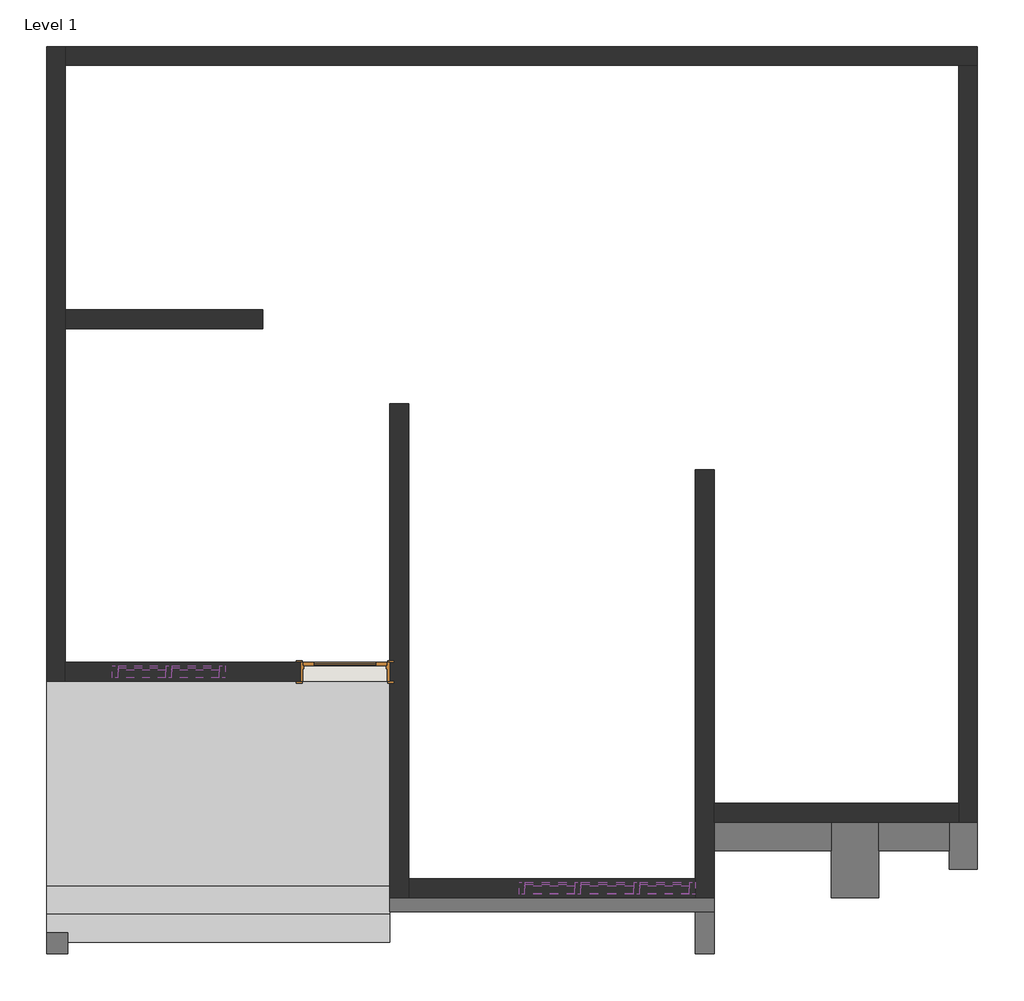
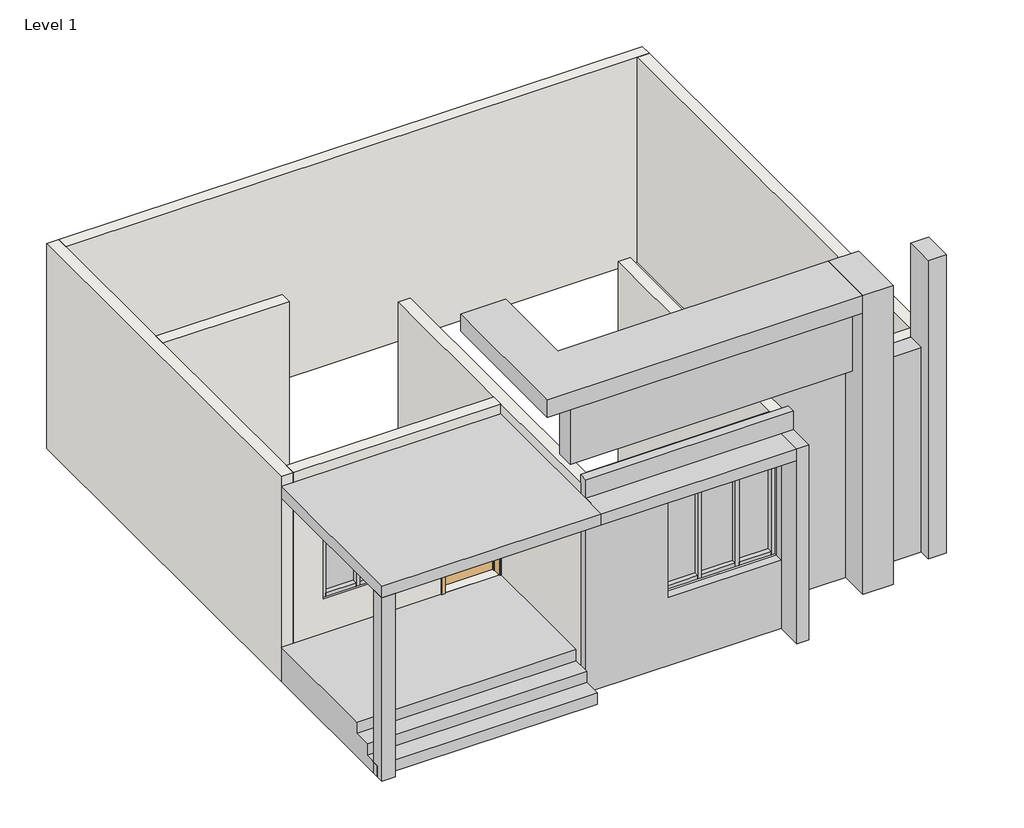
# One storey: 17 members, 9 walls, 5 plates, 1 door, 1 proxy.
"""IFC4 building model written with IfcOpenShell, lengths in millimetres."""

from ifc_helpers import new_model, si_unit, frame, origin, origin_with_axes, place, context, project, spatial, polyline, outline, extrude, faceted_brep, transform, mapped, element, save
from components import generic_models_1_generic_models_1_adbbf048, door_8805718f, member_81de2198, member_d73967ec, member_c8189573, member_bdc0ab2a, member_0b7646a3, system_panel_glazed_2339bcea, system_panel_glazed_76ec949d, system_panel_glazed_5c6be660

model = new_model("IFC4")

# Units and contexts
model_context = context("Model", 3, world=origin())
ifc_project = project(units=[si_unit("LENGTHUNIT", "METRE", prefix="MILLI")], contexts=[model_context])

# Site, building, storey
site = spatial("IfcSite", under=ifc_project)
building = spatial("IfcBuilding", under=site)
storey = spatial("IfcBuildingStorey", under=building, Name="Level 1", Elevation=0.0)

# Proxy
placement = place(None, origin())
generic_models_1_generic_models_1_shape = generic_models_1_generic_models_1_adbbf048(model_context)
element("IfcBuildingElementProxy", 1, Name="Generic Models 1 : Generic Models 1", ObjectType="Generic Models 1 : Generic Models 1", at=placement, inside=storey, context=model_context, shape_type="MappedRepresentation", body=[
    mapped(generic_models_1_generic_models_1_shape, transform((0.0, 0.0, 0.0), x_axis=(1.0, 0.0, 0.0), y_axis=(0.0, 1.0, 0.0), z_axis=(0.0, 0.0, 1.0))),
])

# Door
door_shape = door_8805718f(model_context)
element("IfcDoor", 2, ObjectType="Door-Interior-Single-1_Panel-Wood : 36\" x 96\"", at=placement, inside=storey, context=model_context, shape_type="MappedRepresentation", body=[
    mapped(door_shape, transform((-5421.359401, 7373.8183441, 609.6), x_axis=(1.0, 0.0, 0.0), y_axis=(0.0, 1.0, 0.0), z_axis=(0.0, 0.0, 1.0))),
])

# Members
member_shape = member_81de2198(model_context)
element("IfcMember", 3, ObjectType="Rectangular Mullion : 2.5\" x 5\" rectangular", at=placement, inside=storey, context=model_context, shape_type="MappedRepresentation", body=[
    mapped(member_shape, transform((-3478.259401, 5033.8433441, 3073.4), x_axis=(0.0, 0.0, 1.0), y_axis=(0.0, 1.0, 0.0), z_axis=(-1.0, 0.0, 0.0))),
])
element("IfcMember", 4, ObjectType="Rectangular Mullion : 2.5\" x 5\" rectangular", at=placement, inside=storey, context=model_context, shape_type="MappedRepresentation", body=[
    mapped(member_shape, transform((-2240.009401, 5033.8433441, 3073.4), x_axis=(0.0, 0.0, 1.0), y_axis=(0.0, 1.0, 0.0), z_axis=(-1.0, 0.0, 0.0))),
])
element("IfcMember", 5, ObjectType="Rectangular Mullion : 2.5\" x 5\" rectangular", at=placement, inside=storey, context=model_context, shape_type="MappedRepresentation", body=[
    mapped(member_shape, transform((-1700.259401, 5033.8433441, 1219.2), x_axis=(0.0, 0.0, -1.0), y_axis=(0.0, 1.0, 0.0), z_axis=(1.0, 0.0, 0.0))),
])
element("IfcMember", 6, ObjectType="Rectangular Mullion : 2.5\" x 5\" rectangular", at=placement, inside=storey, context=model_context, shape_type="MappedRepresentation", body=[
    mapped(member_shape, transform((-2938.509401, 5033.8433441, 1219.2), x_axis=(0.0, 0.0, -1.0), y_axis=(0.0, 1.0, 0.0), z_axis=(1.0, 0.0, 0.0))),
])
member_2_shape = member_d73967ec(model_context)
element("IfcMember", 7, ObjectType="Rectangular Mullion : 2.5\" x 5\" rectangular", at=placement, inside=storey, context=model_context, shape_type="MappedRepresentation", body=[
    mapped(member_2_shape, transform((-2906.759401, 5033.8433441, 1219.2), x_axis=(-1.0, 0.0, 0.0), y_axis=(0.0, 1.0, 0.0), z_axis=(0.0, 0.0, -1.0))),
])
element("IfcMember", 8, ObjectType="Rectangular Mullion : 2.5\" x 5\" rectangular", at=placement, inside=storey, context=model_context, shape_type="MappedRepresentation", body=[
    mapped(member_2_shape, transform((-2271.759401, 5033.8433441, 1219.2), x_axis=(-1.0, 0.0, 0.0), y_axis=(0.0, 1.0, 0.0), z_axis=(0.0, 0.0, -1.0))),
])
member_3_shape = member_c8189573(model_context)
element("IfcMember", 9, ObjectType="Rectangular Mullion : 2.5\" x 5\" rectangular", at=placement, inside=storey, context=model_context, shape_type="MappedRepresentation", body=[
    mapped(member_3_shape, transform((-2303.509401, 5033.8433441, 1219.2), x_axis=(0.0, 0.0, -1.0), y_axis=(0.0, 1.0, 0.0), z_axis=(1.0, 0.0, 0.0))),
])
element("IfcMember", 10, ObjectType="Rectangular Mullion : 2.5\" x 5\" rectangular", at=placement, inside=storey, context=model_context, shape_type="MappedRepresentation", body=[
    mapped(member_3_shape, transform((-2875.009401, 5033.8433441, 3073.4), x_axis=(0.0, 0.0, 1.0), y_axis=(0.0, 1.0, 0.0), z_axis=(-1.0, 0.0, 0.0))),
])
member_4_shape = member_bdc0ab2a(model_context)
element("IfcMember", 11, ObjectType="Rectangular Mullion : 2.5\" x 5\" rectangular", at=placement, inside=storey, context=model_context, shape_type="MappedRepresentation", body=[
    mapped(member_4_shape, transform((-1636.759401, 5033.8433441, 3073.4), x_axis=(1.0, 0.0, 0.0), y_axis=(0.0, 1.0, 0.0), z_axis=(0.0, 0.0, 1.0))),
])
element("IfcMember", 12, ObjectType="Rectangular Mullion : 2.5\" x 5\" rectangular", at=placement, inside=storey, context=model_context, shape_type="MappedRepresentation", body=[
    mapped(member_4_shape, transform((-3541.759401, 5033.8433441, 1219.2), x_axis=(-1.0, 0.0, 0.0), y_axis=(0.0, 1.0, 0.0), z_axis=(0.0, 0.0, -1.0))),
])
member_5_shape = member_0b7646a3(model_context)
element("IfcMember", 13, ObjectType="Rectangular Mullion : 2.5\" x 5\" rectangular", at=placement, inside=storey, context=model_context, shape_type="MappedRepresentation", body=[
    mapped(member_5_shape, transform((-6780.259401, 7370.6433441, 3073.4), x_axis=(0.0, 0.0, 1.0), y_axis=(0.0, -1.0, 0.0), z_axis=(1.0, 0.0, 0.0))),
])
element("IfcMember", 14, ObjectType="Rectangular Mullion : 2.5\" x 5\" rectangular", at=placement, inside=storey, context=model_context, shape_type="MappedRepresentation", body=[
    mapped(member_5_shape, transform((-7358.109401, 7370.6433441, 3073.4), x_axis=(0.0, 0.0, 1.0), y_axis=(0.0, -1.0, 0.0), z_axis=(1.0, 0.0, 0.0))),
])
element("IfcMember", 15, ObjectType="Rectangular Mullion : 2.5\" x 5\" rectangular", at=placement, inside=storey, context=model_context, shape_type="MappedRepresentation", body=[
    mapped(member_5_shape, transform((-7872.459401, 7370.6433441, 1219.2), x_axis=(0.0, 0.0, -1.0), y_axis=(0.0, -1.0, 0.0), z_axis=(-1.0, 0.0, 0.0))),
])
element("IfcMember", 16, ObjectType="Rectangular Mullion : 2.5\" x 5\" rectangular", at=placement, inside=storey, context=model_context, shape_type="MappedRepresentation", body=[
    mapped(member_5_shape, transform((-7294.609401, 7370.6433441, 1219.2), x_axis=(0.0, 0.0, -1.0), y_axis=(0.0, -1.0, 0.0), z_axis=(-1.0, 0.0, 0.0))),
])
element("IfcMember", 17, ObjectType="Rectangular Mullion : 2.5\" x 5\" rectangular", at=placement, inside=storey, context=model_context, shape_type="MappedRepresentation", body=[
    mapped(member_2_shape, transform((-7326.359401, 7370.6433441, 1219.2), x_axis=(1.0, 0.0, 0.0), y_axis=(0.0, -1.0, 0.0), z_axis=(0.0, 0.0, -1.0))),
])
element("IfcMember", 18, ObjectType="Rectangular Mullion : 2.5\" x 5\" rectangular", at=placement, inside=storey, context=model_context, shape_type="MappedRepresentation", body=[
    mapped(member_4_shape, transform((-7935.959401, 7370.6433441, 3073.4), x_axis=(-1.0, 0.0, 0.0), y_axis=(0.0, -1.0, 0.0), z_axis=(0.0, 0.0, 1.0))),
])
element("IfcMember", 19, ObjectType="Rectangular Mullion : 2.5\" x 5\" rectangular", at=placement, inside=storey, context=model_context, shape_type="MappedRepresentation", body=[
    mapped(member_4_shape, transform((-6716.759401, 7370.6433441, 1219.2), x_axis=(1.0, 0.0, 0.0), y_axis=(0.0, -1.0, 0.0), z_axis=(0.0, 0.0, -1.0))),
])

# Plates
system_panel_glazed_shape = system_panel_glazed_2339bcea(model_context)
element("IfcPlate", 20, ObjectType="System Panel : Glazed", at=placement, inside=storey, context=model_context, shape_type="MappedRepresentation", body=[
    mapped(system_panel_glazed_shape, transform((-1970.134401, 5033.8433441, 1282.7), x_axis=(-1.0, 0.0, 0.0), y_axis=(0.0, -1.0, 0.0), z_axis=(0.0, 0.0, 1.0))),
])
element("IfcPlate", 21, ObjectType="System Panel : Glazed", at=placement, inside=storey, context=model_context, shape_type="MappedRepresentation", body=[
    mapped(system_panel_glazed_shape, transform((-3208.384401, 5033.8433441, 1282.7), x_axis=(-1.0, 0.0, 0.0), y_axis=(0.0, -1.0, 0.0), z_axis=(0.0, 0.0, 1.0))),
])
system_panel_glazed_2_shape = system_panel_glazed_76ec949d(model_context)
element("IfcPlate", 22, ObjectType="System Panel : Glazed", at=placement, inside=storey, context=model_context, shape_type="MappedRepresentation", body=[
    mapped(system_panel_glazed_2_shape, transform((-2589.259401, 5033.8433441, 1282.7), x_axis=(-1.0, 0.0, 0.0), y_axis=(0.0, -1.0, 0.0), z_axis=(0.0, 0.0, 1.0))),
])
system_panel_glazed_3_shape = system_panel_glazed_5c6be660(model_context)
element("IfcPlate", 23, ObjectType="System Panel : Glazed", at=placement, inside=storey, context=model_context, shape_type="MappedRepresentation", body=[
    mapped(system_panel_glazed_3_shape, transform((-7615.284401, 7370.6433441, 1282.7), x_axis=(1.0, 0.0, 0.0), y_axis=(0.0, 1.0, 0.0), z_axis=(0.0, 0.0, 1.0))),
])
element("IfcPlate", 24, ObjectType="System Panel : Glazed", at=placement, inside=storey, context=model_context, shape_type="MappedRepresentation", body=[
    mapped(system_panel_glazed_3_shape, transform((-7037.434401, 7370.6433441, 1282.7), x_axis=(1.0, 0.0, 0.0), y_axis=(0.0, 1.0, 0.0), z_axis=(0.0, 0.0, 1.0))),
])

# Walls
element("IfcWall", 25, ObjectType="9\" wall", at=placement, inside=storey, context=model_context, shape_type="Brep", body=[
    faceted_brep([(-8647.159401, 14127.0433441, 0.0), (-8647.159401, 7269.0433441, 0.0), (-8647.159401, 7269.0433441, 3657.6), (-8647.159401, 14127.0433441, 3657.6), (-8443.959401, 14127.0433441, 0.0), (-8443.959401, 14127.0433441, 3657.6), (-8443.959401, 13923.8433441, 3657.6), (-8443.959401, 11282.2433441, 3657.6), (-8443.959401, 11079.0433441, 3657.6), (-8443.959401, 7472.2433441, 3657.6), (-8443.959401, 7269.0433441, 3657.6), (-8443.959401, 7269.0433441, 0.0), (-8443.959401, 7472.2433441, 0.0), (-8443.959401, 11079.0433441, 0.0), (-8443.959401, 11282.2433441, 0.0), (-8443.959401, 13923.8433441, 0.0)], [[[0, 1, 2, 3]], [[4, 5, 6, 7, 8, 9, 10, 11, 12, 13, 14, 15]], [[1, 0, 4, 15, 14, 13, 12, 11]], [[3, 2, 10, 9, 8, 7, 6, 5]], [[2, 1, 11, 10]], [[0, 3, 5, 4]]]),
])
element("IfcWall", 26, ObjectType="9\" wall", at=placement, inside=storey, context=model_context, shape_type="SweptSolid", body=[
    extrude(outline(polyline([(-6310.359401, 11079.0433441), (-8443.959401, 11079.0433441), (-8443.959401, 11282.2433441), (-6310.359401, 11282.2433441), (-6310.359401, 11079.0433441)])), origin_with_axes(), (0.0, 0.0, 1.0), 3657.6),
])
element("IfcWall", 27, ObjectType="9\" wall", at=placement, inside=storey, context=model_context, shape_type="SweptSolid", body=[
    extrude(outline(polyline([(0.0, -8443.959401), (0.0, -4938.759401), (609.6, -4938.759401), (609.6, -5903.959401), (3073.4, -5903.959401), (3073.4, -4938.759401), (3657.6, -4938.759401), (3657.6, -8443.959401), (0.0, -8443.959401)]), holes=[polyline([(1219.2, -7935.959401), (3073.4, -7935.959401), (3073.4, -6716.759401), (1219.2, -6716.759401), (1219.2, -7935.959401)])]), frame((0.0, 7269.0433441, 0.0), z_axis=(0.0, 1.0, 0.0), x_axis=(0.0, 0.0, 1.0)), (0.0, 0.0, 1.0), 203.2),
])
element("IfcWall", 28, ObjectType="9\" wall", at=placement, inside=storey, context=model_context, shape_type="Brep", body=[
    faceted_brep([(-8443.959401, 13923.8433441, 0.0), (1208.040599, 13923.8433441, 0.0), (1411.240599, 13923.8433441, 0.0), (1411.240599, 13923.8433441, 3657.6), (1208.040599, 13923.8433441, 3657.6), (-8443.959401, 13923.8433441, 3657.6), (-8443.959401, 14127.0433441, 0.0), (-8443.959401, 14127.0433441, 3657.6), (1411.240599, 14127.0433441, 3657.6), (1411.240599, 14127.0433441, 0.0)], [[[0, 1, 2, 3, 4, 5]], [[6, 7, 8, 9]], [[2, 1, 0, 6, 9]], [[5, 4, 3, 8, 7]], [[0, 5, 7, 6]], [[3, 2, 9, 8]]]),
])
element("IfcWall", 29, ObjectType="9\" wall", at=placement, inside=storey, context=model_context, shape_type="Brep", body=[
    faceted_brep([(1208.040599, 13923.8433441, 0.0), (1208.040599, 5948.2433441, 0.0), (1208.040599, 5745.0433441, 0.0), (1208.040599, 5745.0433441, 3657.6), (1208.040599, 5948.2433441, 3657.6), (1208.040599, 13923.8433441, 3657.6), (1411.240599, 13923.8433441, 0.0), (1411.240599, 13923.8433441, 3657.6), (1411.240599, 5745.0433441, 3657.6), (1411.240599, 5745.0433441, 0.0)], [[[0, 1, 2, 3, 4, 5]], [[6, 7, 8, 9]], [[2, 1, 0, 6, 9]], [[5, 4, 3, 8, 7]], [[0, 5, 7, 6]], [[3, 2, 9, 8]]]),
])
element("IfcWall", 30, ObjectType="9\" wall", at=placement, inside=storey, context=model_context, shape_type="SweptSolid", body=[
    extrude(outline(polyline([(-1433.559401, 5948.2433441), (1208.040599, 5948.2433441), (1208.040599, 5745.0433441), (-1433.559401, 5745.0433441), (-1433.559401, 5948.2433441)])), origin_with_axes(), (0.0, 0.0, 1.0), 3657.6),
])
element("IfcWall", 31, ObjectType="9\" wall", at=placement, inside=storey, context=model_context, shape_type="Brep", body=[
    faceted_brep([(-1433.559401, 4932.2433441, 0.0), (-1433.559401, 5745.0433441, 0.0), (-1433.559401, 5948.2433441, 0.0), (-1433.559401, 9555.0433441, 0.0), (-1433.559401, 9555.0433441, 3657.6), (-1433.559401, 5948.2433441, 3657.6), (-1433.559401, 5745.0433441, 3657.6), (-1433.559401, 4932.2433441, 3657.6), (-1636.759401, 4932.2433441, 0.0), (-1636.759401, 4932.2433441, 1219.2), (-1636.759401, 4932.2433441, 3073.4), (-1636.759401, 4932.2433441, 3657.6), (-1636.759401, 5135.4433441, 3657.6), (-1636.759401, 9555.0433441, 3657.6), (-1636.759401, 9555.0433441, 0.0), (-1636.759401, 5135.4433441, 0.0)], [[[0, 1, 2, 3, 4, 5, 6, 7]], [[8, 9, 10, 11, 12, 13, 14, 15]], [[3, 2, 1, 0, 8, 15, 14]], [[4, 3, 14, 13]], [[7, 6, 5, 4, 13, 12, 11]], [[0, 7, 11, 10, 9, 8]]]),
])
element("IfcWall", 32, ObjectType="9\" wall", at=placement, inside=storey, context=model_context, shape_type="Brep", body=[
    faceted_brep([(-4938.759401, 10266.2433441, 0.0), (-4938.759401, 7472.2433441, 0.0), (-4938.759401, 7269.0433441, 0.0), (-4938.759401, 4932.2433441, 0.0), (-4938.759401, 4932.2433441, 3657.6), (-4938.759401, 7269.0433441, 3657.6), (-4938.759401, 7472.2433441, 3657.6), (-4938.759401, 10266.2433441, 3657.6), (-4735.559401, 10266.2433441, 0.0), (-4735.559401, 10266.2433441, 3657.6), (-4735.559401, 5135.4433441, 3657.6), (-4735.559401, 4932.2433441, 3657.6), (-4735.559401, 4932.2433441, 0.0), (-4735.559401, 5135.4433441, 0.0)], [[[0, 1, 2, 3, 4, 5, 6, 7]], [[8, 9, 10, 11, 12, 13]], [[3, 2, 1, 0, 8, 13, 12]], [[7, 6, 5, 4, 11, 10, 9]], [[0, 7, 9, 8]], [[4, 3, 12, 11]]]),
])
element("IfcWall", 33, ObjectType="9\" wall", at=placement, inside=storey, context=model_context, shape_type="SweptSolid", body=[
    extrude(outline(polyline([(0.0, -4735.559401), (0.0, -1636.759401), (1219.2, -1636.759401), (1219.2, -3541.759401), (3073.4, -3541.759401), (3073.4, -1636.759401), (3657.6, -1636.759401), (3657.6, -4735.559401), (0.0, -4735.559401)])), frame((0.0, 4932.2433441, 0.0), z_axis=(0.0, 1.0, 0.0), x_axis=(0.0, 0.0, 1.0)), (0.0, 0.0, 1.0), 203.2),
])

save(model, "model.ifc")

# Revit data of these elements
# Type "Door-Interior-Single-1_Panel-Wood : 36\" x 96\""
#   Type Mark = "8"
#   Assembly Code = "C1020300"
#   Analytic Construction = "Wooden"
#   Top Rail = 0' - 4 11/16"
#   Thickness = 0' - 1 3/8"
#   Thermal Resistance (R) = 2.5876 (h·ft²·°F)/BTU
#   Swing Angle [instance default] = 90.00°
#   Stiles = 0' - 4 3/4"
#   Rough Width = 3' - 2"
#   Rough Height = 8' - 1"
#   Height = 8' - 0"
#   Width = 3' - 0"
#   Heat Transfer Coefficient (U) = 0.3865 BTU/(h·ft²·°F)
#   Bottom Rail = 0' - 9 1/8"
#   Trim Material = Cherry
#   Panel Material = Cherry
#   Frame Material = Cherry
#   Door Handle Material = Aluminum
#   Visual Light Transmittance = 0
#   Solar Heat Gain Coefficient = 0
#   Wall Closure = (empty or 0)
#   Function = (empty or 0)
# Type "Rectangular Mullion : 2.5\" x 5\" rectangular"
#   built-in parameter 1007304 = 0.416667 (stored number, unit not read)
#   built-in parameter 1007301 = 0.104167 (stored number, unit not read)
#   built-in parameter 1007300 = 0.104167 (stored number, unit not read)
# Type "System Panel : Glazed"
#   Construction Type Id = "GSP4R"
#   Analytic Construction = "1/8 in Pilkington single glazing"
#   Visual Light Transmittance = 0.9
#   Solar Heat Gain Coefficient = 0.86
#   Heat Transfer Coefficient (U) = 1.18115 BTU/(h·ft²·°F)
#   Define Thermal Properties by = 1
# Type "9\" wall"
#   Assembly Code = "B2010"
#   Layers, outside or top first: 0' - 8" no material (function 1)
# Element 1 (IfcBuildingElementProxy, "Generic Models 1 : Generic Models 1")
#   Phase Created = New Construction
# Element 2 (IfcDoor, "Door-Interior-Single-1_Panel-Wood : 36\" x 96\"")
#   Swing Angle = 90.00°
#   Phase Created = New Construction
#   Materials on its faces: "Cherry", "Aluminum"
# Elements 3, 4, 5, 6, 7, 8, 9, 10, 11, 12, 13, 14, 15, 16, 17, 18, 19 (IfcMember, "Rectangular Mullion : 2.5\" x 5\" rectangular")
#   Phase Created = New Construction
#   Materials on its faces: "Aluminum"
# Elements 20, 21, 22, 23, 24 (IfcPlate, "System Panel : Glazed")
#   Phase Created = New Construction
#   Materials on its faces: "Glass"
# Elements 25, 26, 27, 28, 29, 30, 31, 32, 33 (IfcWall, "9\" wall")
#   Top Offset = 0' - 0"
#   Base Offset = 0' - 0"
#   wall height = 12' - 0"
#   Phase Created = New Construction
#   Base Constraint = Level 1
#   Top Constraint = Level 3
#   Materials on its faces: "Default Wall"
# Materials
#   "Cherry": class "Wood", colour RGB 226 177 128, transparency 0, Description = "Prunus Serotina", Cost = 0
#   "Aluminum": class "Metal", colour RGB 247 247 247, transparency 0, Description = "Aluminum 6061", Cost = 0
#   "Glass": class "Glass", colour RGB 0 128 192, transparency 0.75, Description = "Soda Lime Glass", Cost = 0
#   "Default Wall": colour RGB 128 128 128, transparency 0, Cost = 0
